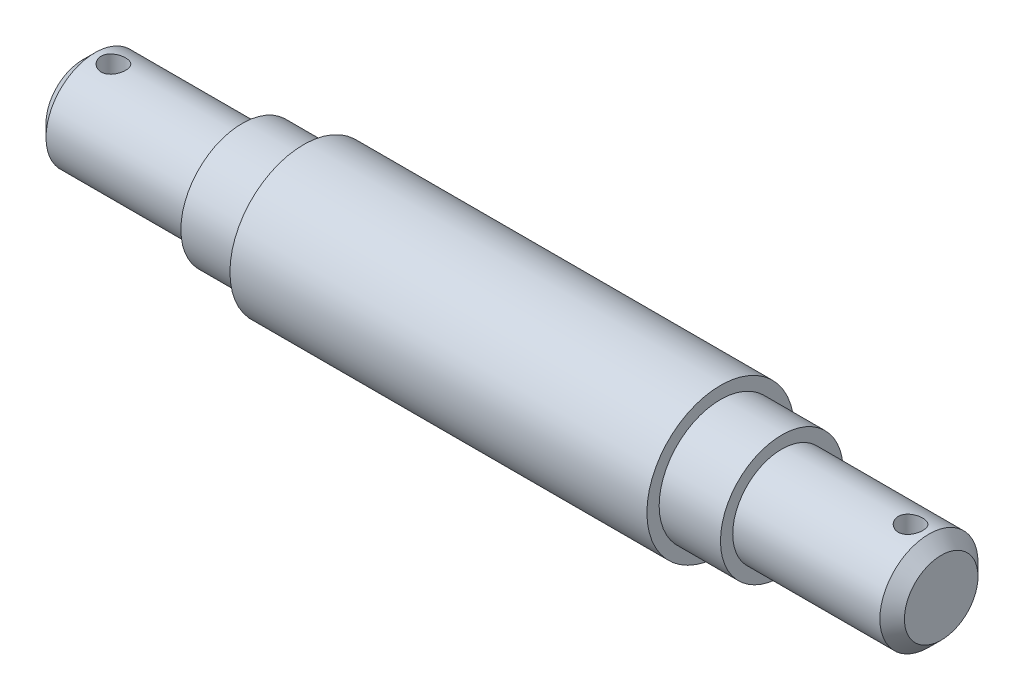
ISO-10303-21;
HEADER;
FILE_DESCRIPTION(('STEP AP214'),'2;1');
FILE_NAME('part.step','',(''),(''),'','','');
FILE_SCHEMA(('AUTOMOTIVE_DESIGN { 1 0 10303 214 1 1 1 1 }'));
ENDSEC;
DATA;
#1=APPLICATION_CONTEXT('core data for automotive mechanical design processes');
#2=APPLICATION_PROTOCOL_DEFINITION('international standard','automotive_design',2000,#1);
#3=PRODUCT_CONTEXT('',#1,'mechanical');
#4=PRODUCT('Part','Part','',(#3));
#5=PRODUCT_RELATED_PRODUCT_CATEGORY('part','',(#4));
#6=PRODUCT_DEFINITION_FORMATION('','',#4);
#7=PRODUCT_DEFINITION_CONTEXT('part definition',#1,'design');
#8=PRODUCT_DEFINITION('design','',#6,#7);
#9=PRODUCT_DEFINITION_SHAPE('','',#8);
#10=(LENGTH_UNIT() NAMED_UNIT(*) SI_UNIT(.MILLI.,.METRE.));
#11=(NAMED_UNIT(*) PLANE_ANGLE_UNIT() SI_UNIT($,.RADIAN.));
#12=(NAMED_UNIT(*) SI_UNIT($,.STERADIAN.) SOLID_ANGLE_UNIT());
#13=UNCERTAINTY_MEASURE_WITH_UNIT(LENGTH_MEASURE(1.E-05),#10,'distance_accuracy_value','');
#14=(GEOMETRIC_REPRESENTATION_CONTEXT(3) GLOBAL_UNCERTAINTY_ASSIGNED_CONTEXT((#13)) GLOBAL_UNIT_ASSIGNED_CONTEXT((#10,
#11,#12)) REPRESENTATION_CONTEXT('',''));
#15=CARTESIAN_POINT('',(0.,0.,0.));
#16=DIRECTION('',(0.,0.,1.));
#17=DIRECTION('',(1.,0.,0.));
#18=AXIS2_PLACEMENT_3D('',#15,#16,#17);
#19=CARTESIAN_POINT('',(0.,-4.,0.));
#20=DIRECTION('',(-1.,0.,0.));
#21=DIRECTION('',(0.,0.,1.));
#22=AXIS2_PLACEMENT_3D('',#19,#20,#21);
#23=PLANE('',#22);
#24=CARTESIAN_POINT('',(0.,0.,0.));
#25=DIRECTION('',(-1.,0.,0.));
#26=DIRECTION('',(0.,0.,1.));
#27=AXIS2_PLACEMENT_3D('',#24,#25,#26);
#28=CIRCLE('',#27,3.);
#29=CARTESIAN_POINT('',(0.,0.,3.));
#30=VERTEX_POINT('',#29);
#31=EDGE_CURVE('E60',#30,#30,#28,.T.);
#32=ORIENTED_EDGE('',*,*,#31,.T.);
#33=EDGE_LOOP('',(#32));
#34=FACE_BOUND('',#33,.T.);
#35=ADVANCED_FACE('F41',(#34),#23,.T.);
#36=CARTESIAN_POINT('',(70.,0.,0.));
#37=DIRECTION('',(1.,0.,0.));
#38=DIRECTION('',(0.,0.,-1.));
#39=AXIS2_PLACEMENT_3D('',#36,#37,#38);
#40=PLANE('',#39);
#41=CARTESIAN_POINT('',(70.,0.,0.));
#42=DIRECTION('',(1.,0.,0.));
#43=DIRECTION('',(0.,0.,-1.));
#44=AXIS2_PLACEMENT_3D('',#41,#42,#43);
#45=CIRCLE('',#44,3.);
#46=CARTESIAN_POINT('',(70.,0.,-3.));
#47=VERTEX_POINT('',#46);
#48=EDGE_CURVE('E10',#47,#47,#45,.T.);
#49=ORIENTED_EDGE('',*,*,#48,.T.);
#50=EDGE_LOOP('',(#49));
#51=FACE_BOUND('',#50,.T.);
#52=ADVANCED_FACE('F132',(#51),#40,.T.);
#53=CARTESIAN_POINT('',(0.,0.,0.));
#54=DIRECTION('',(-1.,0.,0.));
#55=DIRECTION('',(0.,0.,1.));
#56=AXIS2_PLACEMENT_3D('',#53,#54,#55);
#57=CYLINDRICAL_SURFACE('',#56,4.);
#58=CARTESIAN_POINT('',(69.,0.,0.));
#59=DIRECTION('',(1.,0.,0.));
#60=DIRECTION('',(0.,0.,-1.));
#61=AXIS2_PLACEMENT_3D('',#58,#59,#60);
#62=CIRCLE('',#61,4.);
#63=CARTESIAN_POINT('',(69.,0.,-4.));
#64=VERTEX_POINT('',#63);
#65=EDGE_CURVE('E47',#64,#64,#62,.F.);
#66=ORIENTED_EDGE('',*,*,#65,.T.);
#67=EDGE_LOOP('',(#66));
#68=FACE_BOUND('',#67,.T.);
#69=CARTESIAN_POINT('',(67.5,-3.87298334620742,0.999999999999998));
#70=CARTESIAN_POINT('',(67.4447796996432,-3.87298440057185,0.999998431438697));
#71=CARTESIAN_POINT('',(67.3895420405686,-3.87417722499279,0.995410498208067));
#72=CARTESIAN_POINT('',(67.2806529687674,-3.87880744892249,0.977209250194444));
#73=CARTESIAN_POINT('',(67.22700249822,-3.88224615474181,0.963590682698076));
#74=CARTESIAN_POINT('',(67.1228785847122,-3.89095489813012,0.927796479849631));
#75=CARTESIAN_POINT('',(67.0724011378422,-3.8962225706936,0.905631891140939));
#76=CARTESIAN_POINT('',(66.9758756589875,-3.90799276818327,0.853408456505401));
#77=CARTESIAN_POINT('',(66.9298278151688,-3.91449534553241,0.823349275424499));
#78=CARTESIAN_POINT('',(66.8424553418942,-3.92816286540368,0.755483370924512));
#79=CARTESIAN_POINT('',(66.8012425598597,-3.93533839048709,0.717534755081553));
#80=CARTESIAN_POINT('',(66.7256954422561,-3.94945150206622,0.635272825640327));
#81=CARTESIAN_POINT('',(66.6913617497514,-3.95638906626691,0.590958917672139));
#82=CARTESIAN_POINT('',(66.6300898129474,-3.96936166208095,0.496458080431564));
#83=CARTESIAN_POINT('',(66.6032614447354,-3.975382749602,0.446197830478043));
#84=CARTESIAN_POINT('',(66.5584761423388,-3.98572324770431,0.341705273717105));
#85=CARTESIAN_POINT('',(66.5405178992338,-3.99004290933748,0.28747355431677));
#86=CARTESIAN_POINT('',(66.5143408661686,-3.99641903539263,0.177743503501654));
#87=CARTESIAN_POINT('',(66.5059321422694,-3.99851957537723,0.122293087819583));
#88=CARTESIAN_POINT('',(66.4984966482898,-4.00037437642922,0.0107315277051037));
#89=CARTESIAN_POINT('',(66.4994684911162,-4.00012898438682,-0.0453795178152308));
#90=CARTESIAN_POINT('',(66.5106299401001,-3.99735237981413,-0.15535224717239));
#91=CARTESIAN_POINT('',(66.5206145300216,-3.9948720093635,-0.20923621560107));
#92=CARTESIAN_POINT('',(66.5491885080194,-3.98796334609942,-0.314538247413689));
#93=CARTESIAN_POINT('',(66.567778354151,-3.98353494959376,-0.365956179370442));
#94=CARTESIAN_POINT('',(66.6132010282748,-3.97315003880358,-0.465406703501811));
#95=CARTESIAN_POINT('',(66.6401068178647,-3.96718007878021,-0.513404509766509));
#96=CARTESIAN_POINT('',(66.7013422716465,-3.9543596152386,-0.604275622340492));
#97=CARTESIAN_POINT('',(66.7356732274243,-3.94750895860996,-0.647148035085508));
#98=CARTESIAN_POINT('',(66.811883496793,-3.93345485507808,-0.72777403508496));
#99=CARTESIAN_POINT('',(66.8539419569391,-3.92624687810367,-0.765357679075204));
#100=CARTESIAN_POINT('',(66.9438399894161,-3.91246017406683,-0.832976375963023));
#101=CARTESIAN_POINT('',(66.9916798317964,-3.90588147642388,-0.863011076046019));
#102=CARTESIAN_POINT('',(67.0921160136596,-3.89408198732659,-0.9147881290226));
#103=CARTESIAN_POINT('',(67.1447342921253,-3.88886793490288,-0.936489566970494));
#104=CARTESIAN_POINT('',(67.2530341872306,-3.88047456055983,-0.970685620636343));
#105=CARTESIAN_POINT('',(67.3087151455933,-3.87729480324087,-0.983182206552911));
#106=CARTESIAN_POINT('',(67.4199838006093,-3.87342142415656,-0.998331855466069));
#107=CARTESIAN_POINT('',(67.4755351173319,-3.87266435637459,-1.00123618956785));
#108=CARTESIAN_POINT('',(67.5863287746313,-3.87354937392416,-0.997806796206216));
#109=CARTESIAN_POINT('',(67.6415711431805,-3.87519123840507,-0.991473919139517));
#110=CARTESIAN_POINT('',(67.7492457059819,-3.88062832781824,-0.969970185575061));
#111=CARTESIAN_POINT('',(67.8017090906283,-3.8843878809375,-0.954945627312696));
#112=CARTESIAN_POINT('',(67.9033725831407,-3.89360287308385,-0.916647232668246));
#113=CARTESIAN_POINT('',(67.9525723036221,-3.89905851299446,-0.893372419085015));
#114=CARTESIAN_POINT('',(68.0473765111469,-3.91118454837305,-0.83870826717462));
#115=CARTESIAN_POINT('',(68.0928915360172,-3.91787667442657,-0.80716870153425));
#116=CARTESIAN_POINT('',(68.1780753451205,-3.93166833228686,-0.737060292934454));
#117=CARTESIAN_POINT('',(68.21774316666,-3.93876793091388,-0.698490294805437));
#118=CARTESIAN_POINT('',(68.2911244170284,-3.95278961212643,-0.614262720984723));
#119=CARTESIAN_POINT('',(68.3246640250195,-3.95970280824734,-0.568451952531591));
#120=CARTESIAN_POINT('',(68.3835743467805,-3.97238886645494,-0.471702682694674));
#121=CARTESIAN_POINT('',(68.4089454866433,-3.97816178801584,-0.42076444895759));
#122=CARTESIAN_POINT('',(68.4505784138112,-3.98788046295326,-0.315558201731088));
#123=CARTESIAN_POINT('',(68.4669057137516,-3.99183932008964,-0.261317381027879));
#124=CARTESIAN_POINT('',(68.4901841338434,-3.99754117358315,-0.150749760318804));
#125=CARTESIAN_POINT('',(68.4971370634956,-3.99928459757364,-0.0944233650412395));
#126=CARTESIAN_POINT('',(68.5013675895755,-4.00034169408811,0.0170835264433306));
#127=CARTESIAN_POINT('',(68.4989017090954,-3.99971978880008,0.0722538269660375));
#128=CARTESIAN_POINT('',(68.4849521727057,-3.99625896457423,0.181367496414744));
#129=CARTESIAN_POINT('',(68.4734687849869,-3.99342011157095,0.235310901780891));
#130=CARTESIAN_POINT('',(68.4419477802291,-3.98585432853963,0.34017103564482));
#131=CARTESIAN_POINT('',(68.4219565466854,-3.98113764502669,0.391102494581023));
#132=CARTESIAN_POINT('',(68.3740294209807,-3.97031288913382,0.488917053041472));
#133=CARTESIAN_POINT('',(68.3460925273304,-3.96420464137727,0.535799641265055));
#134=CARTESIAN_POINT('',(68.2822847660029,-3.95107249681342,0.625401928423903));
#135=CARTESIAN_POINT('',(68.2462398570926,-3.94403016945647,0.667994988300589));
#136=CARTESIAN_POINT('',(68.1675771480262,-3.92990649053207,0.746615020271253));
#137=CARTESIAN_POINT('',(68.1249576839021,-3.92282512952424,0.782640325068179));
#138=CARTESIAN_POINT('',(68.0333985857987,-3.90927475860683,0.847762026479241));
#139=CARTESIAN_POINT('',(67.9843558765875,-3.90281963730391,0.876716619446593));
#140=CARTESIAN_POINT('',(67.8819445100771,-3.8914395555011,0.925926896615621));
#141=CARTESIAN_POINT('',(67.8285790338927,-3.88651348244814,0.946188909759556));
#142=CARTESIAN_POINT('',(67.7294229881737,-3.87951908741315,0.97442252856557));
#143=CARTESIAN_POINT('',(67.6841068356177,-3.87708663005761,0.983993170595826));
#144=CARTESIAN_POINT('',(67.5925311309985,-3.87381838580358,0.996782292572817));
#145=CARTESIAN_POINT('',(67.5462716597494,-3.87298246270639,1.00000131437052));
#146=CARTESIAN_POINT('',(67.5,-3.87298334620742,0.999999999999998));
#147=B_SPLINE_CURVE_WITH_KNOTS('',3,(#69,#70,#71,#72,#73,#74,#75,#76,#77,#78,#79,#80,#81,#82,
#83,#84,#85,#86,#87,#88,#89,#90,#91,#92,#93,#94,#95,#96,#97,#98,#99,#100,#101,#102,#103,#104,
#105,#106,#107,#108,#109,#110,#111,#112,#113,#114,#115,#116,#117,#118,#119,#120,#121,#122,#123,
#124,#125,#126,#127,#128,#129,#130,#131,#132,#133,#134,#135,#136,#137,#138,#139,#140,#141,#142,
#143,#144,#145,#146),.UNSPECIFIED.,.T.,.F.,(4,2,2,2,2,2,2,2,2,2,2,2,2,2,2,2,2,2,2,2,2,2,2,2,2,2,
2,2,2,2,2,2,2,2,2,2,2,2,4),(0.,0.165490976675223,0.331078296534215,0.496452290829154,
0.661833306984669,0.830495816734641,0.999174085882202,1.17020598555443,1.34121263935112,
1.50875500394413,1.67627259462682,1.84007305071853,2.00388222686189,2.16917149698053,
2.33448954183839,2.50428186625039,2.67408212476195,2.84470572799637,3.01529280048094,
3.18137429900961,3.34744050869796,3.51078961999956,3.6741580856484,3.84073138339936,
4.00733207550291,4.17810132382401,4.34886166284094,4.51836829119045,4.68784219559889,
4.85273378447256,5.01762046947066,5.18161950620158,5.34563922291503,5.51358838629102,
5.68158012622477,5.85270590910144,6.02370688542921,6.16239130867204,6.30106390036081),.UNSPECIFIED.);
#148=CARTESIAN_POINT('',(67.5,-3.87298334620742,0.999999999999998));
#149=VERTEX_POINT('',#148);
#150=EDGE_CURVE('E62',#149,#149,#147,.T.);
#151=ORIENTED_EDGE('',*,*,#150,.F.);
#152=EDGE_LOOP('',(#151));
#153=FACE_BOUND('',#152,.T.);
#154=CARTESIAN_POINT('',(67.5,3.87298334620742,0.999999999999998));
#155=CARTESIAN_POINT('',(67.5552203003568,3.87298440057185,0.999998431438697));
#156=CARTESIAN_POINT('',(67.6104579594314,3.87417722499279,0.995410498208067));
#157=CARTESIAN_POINT('',(67.7193470312326,3.87880744892249,0.977209250194444));
#158=CARTESIAN_POINT('',(67.77299750178,3.88224615474181,0.963590682698076));
#159=CARTESIAN_POINT('',(67.8771214152878,3.89095489813012,0.927796479849631));
#160=CARTESIAN_POINT('',(67.9275988621578,3.8962225706936,0.905631891140939));
#161=CARTESIAN_POINT('',(68.0241243410125,3.90799276818327,0.853408456505401));
#162=CARTESIAN_POINT('',(68.0701721848312,3.91449534553241,0.823349275424499));
#163=CARTESIAN_POINT('',(68.1575446581058,3.92816286540368,0.755483370924512));
#164=CARTESIAN_POINT('',(68.1987574401403,3.93533839048709,0.717534755081553));
#165=CARTESIAN_POINT('',(68.2743045577439,3.94945150206622,0.635272825640327));
#166=CARTESIAN_POINT('',(68.3086382502486,3.95638906626691,0.590958917672139));
#167=CARTESIAN_POINT('',(68.3699101870526,3.96936166208095,0.496458080431564));
#168=CARTESIAN_POINT('',(68.3967385552646,3.975382749602,0.446197830478043));
#169=CARTESIAN_POINT('',(68.4415238576612,3.98572324770431,0.341705273717105));
#170=CARTESIAN_POINT('',(68.4594821007662,3.99004290933748,0.28747355431677));
#171=CARTESIAN_POINT('',(68.4856591338314,3.99641903539263,0.177743503501654));
#172=CARTESIAN_POINT('',(68.4940678577306,3.99851957537723,0.122293087819583));
#173=CARTESIAN_POINT('',(68.5015033517102,4.00037437642922,0.0107315277051038));
#174=CARTESIAN_POINT('',(68.5005315088838,4.00012898438682,-0.0453795178152307));
#175=CARTESIAN_POINT('',(68.4893700598999,3.99735237981413,-0.15535224717239));
#176=CARTESIAN_POINT('',(68.4793854699785,3.9948720093635,-0.20923621560107));
#177=CARTESIAN_POINT('',(68.4508114919806,3.98796334609942,-0.314538247413689));
#178=CARTESIAN_POINT('',(68.432221645849,3.98353494959376,-0.365956179370441));
#179=CARTESIAN_POINT('',(68.3867989717252,3.97315003880358,-0.465406703501808));
#180=CARTESIAN_POINT('',(68.3598931821353,3.96718007878021,-0.513404509766505));
#181=CARTESIAN_POINT('',(68.2986577283535,3.9543596152386,-0.604275622340489));
#182=CARTESIAN_POINT('',(68.2643267725758,3.94750895860996,-0.647148035085506));
#183=CARTESIAN_POINT('',(68.1881165032071,3.93345485507808,-0.727774035084959));
#184=CARTESIAN_POINT('',(68.1460580430609,3.92624687810367,-0.765357679075204));
#185=CARTESIAN_POINT('',(68.0561600105839,3.91246017406682,-0.832976375963023));
#186=CARTESIAN_POINT('',(68.0083201682036,3.90588147642388,-0.863011076046019));
#187=CARTESIAN_POINT('',(67.9078839863404,3.89408198732659,-0.914788129022598));
#188=CARTESIAN_POINT('',(67.8552657078747,3.88886793490288,-0.936489566970491));
#189=CARTESIAN_POINT('',(67.7469658127694,3.88047456055983,-0.970685620636341));
#190=CARTESIAN_POINT('',(67.6912848544067,3.87729480324087,-0.98318220655291));
#191=CARTESIAN_POINT('',(67.5800161993907,3.87342142415656,-0.998331855466069));
#192=CARTESIAN_POINT('',(67.5244648826681,3.87266435637459,-1.00123618956785));
#193=CARTESIAN_POINT('',(67.4136712253687,3.87354937392416,-0.997806796206216));
#194=CARTESIAN_POINT('',(67.3584288568195,3.87519123840507,-0.991473919139516));
#195=CARTESIAN_POINT('',(67.2507542940181,3.88062832781824,-0.96997018557506));
#196=CARTESIAN_POINT('',(67.1982909093717,3.8843878809375,-0.954945627312694));
#197=CARTESIAN_POINT('',(67.0966274168593,3.89360287308385,-0.916647232668243));
#198=CARTESIAN_POINT('',(67.0474276963779,3.89905851299446,-0.893372419085012));
#199=CARTESIAN_POINT('',(66.9526234888531,3.91118454837305,-0.83870826717462));
#200=CARTESIAN_POINT('',(66.9071084639828,3.91787667442657,-0.80716870153425));
#201=CARTESIAN_POINT('',(66.8219246548795,3.93166833228686,-0.737060292934454));
#202=CARTESIAN_POINT('',(66.78225683334,3.93876793091388,-0.698490294805437));
#203=CARTESIAN_POINT('',(66.7088755829716,3.95278961212643,-0.614262720984723));
#204=CARTESIAN_POINT('',(66.6753359749805,3.95970280824734,-0.568451952531591));
#205=CARTESIAN_POINT('',(66.6164256532195,3.97238886645494,-0.471702682694674));
#206=CARTESIAN_POINT('',(66.5910545133567,3.97816178801584,-0.42076444895759));
#207=CARTESIAN_POINT('',(66.5494215861888,3.98788046295326,-0.315558201731088));
#208=CARTESIAN_POINT('',(66.5330942862484,3.99183932008964,-0.261317381027879));
#209=CARTESIAN_POINT('',(66.5098158661566,3.99754117358315,-0.150749760318804));
#210=CARTESIAN_POINT('',(66.5028629365044,3.99928459757364,-0.0944233650412395));
#211=CARTESIAN_POINT('',(66.4986324104245,4.00034169408811,0.0170835264433306));
#212=CARTESIAN_POINT('',(66.5010982909046,3.99971978880008,0.0722538269660375));
#213=CARTESIAN_POINT('',(66.5150478272943,3.99625896457423,0.181367496414744));
#214=CARTESIAN_POINT('',(66.5265312150131,3.99342011157095,0.235310901780891));
#215=CARTESIAN_POINT('',(66.5580522197709,3.98585432853963,0.34017103564482));
#216=CARTESIAN_POINT('',(66.5780434533146,3.98113764502669,0.391102494581023));
#217=CARTESIAN_POINT('',(66.6259705790193,3.97031288913382,0.488917053041472));
#218=CARTESIAN_POINT('',(66.6539074726696,3.96420464137727,0.535799641265055));
#219=CARTESIAN_POINT('',(66.7177152339971,3.95107249681342,0.625401928423903));
#220=CARTESIAN_POINT('',(66.7537601429074,3.94403016945647,0.667994988300589));
#221=CARTESIAN_POINT('',(66.8324228519738,3.92990649053207,0.746615020271253));
#222=CARTESIAN_POINT('',(66.8750423160979,3.92282512952424,0.782640325068179));
#223=CARTESIAN_POINT('',(66.9666014142013,3.90927475860683,0.847762026479241));
#224=CARTESIAN_POINT('',(67.0156441234125,3.90281963730391,0.876716619446593));
#225=CARTESIAN_POINT('',(67.1180554899229,3.8914395555011,0.925926896615621));
#226=CARTESIAN_POINT('',(67.1714209661073,3.88651348244814,0.946188909759556));
#227=CARTESIAN_POINT('',(67.2705770118263,3.87951908741315,0.97442252856557));
#228=CARTESIAN_POINT('',(67.3158931643824,3.87708663005761,0.983993170595826));
#229=CARTESIAN_POINT('',(67.4074688690015,3.87381838580358,0.996782292572817));
#230=CARTESIAN_POINT('',(67.4537283402506,3.87298246270639,1.00000131437052));
#231=CARTESIAN_POINT('',(67.5,3.87298334620742,0.999999999999998));
#232=B_SPLINE_CURVE_WITH_KNOTS('',3,(#154,#155,#156,#157,#158,#159,#160,#161,#162,#163,#164,
#165,#166,#167,#168,#169,#170,#171,#172,#173,#174,#175,#176,#177,#178,#179,#180,#181,#182,#183,
#184,#185,#186,#187,#188,#189,#190,#191,#192,#193,#194,#195,#196,#197,#198,#199,#200,#201,#202,
#203,#204,#205,#206,#207,#208,#209,#210,#211,#212,#213,#214,#215,#216,#217,#218,#219,#220,#221,
#222,#223,#224,#225,#226,#227,#228,#229,#230,#231),.UNSPECIFIED.,.T.,.F.,(4,2,2,2,2,2,2,2,2,2,2,
2,2,2,2,2,2,2,2,2,2,2,2,2,2,2,2,2,2,2,2,2,2,2,2,2,2,2,4),(0.,0.165490976675223,
0.331078296534215,0.496452290829154,0.661833306984669,0.830495816734641,0.999174085882202,
1.17020598555443,1.34121263935112,1.50875500394413,1.67627259462682,1.84007305071853,
2.00388222686189,2.16917149698051,2.33448954183839,2.50428186625039,2.67408212476196,
2.84470572799636,3.01529280048094,3.18137429900961,3.34744050869796,3.51078961999957,
3.6741580856484,3.84073138339937,4.00733207550291,4.17810132382402,4.34886166284095,
4.51836829119045,4.68784219559889,4.85273378447256,5.01762046947066,5.18161950620158,
5.34563922291503,5.51358838629102,5.68158012622477,5.85270590910144,6.02370688542921,
6.16239130867204,6.30106390036081),.UNSPECIFIED.);
#233=CARTESIAN_POINT('',(67.5,3.87298334620742,0.999999999999998));
#234=VERTEX_POINT('',#233);
#235=EDGE_CURVE('E75',#234,#234,#232,.T.);
#236=ORIENTED_EDGE('',*,*,#235,.F.);
#237=EDGE_LOOP('',(#236));
#238=FACE_BOUND('',#237,.T.);
#239=CARTESIAN_POINT('',(57.,0.,0.));
#240=DIRECTION('',(-1.,0.,0.));
#241=DIRECTION('',(0.,0.,1.));
#242=AXIS2_PLACEMENT_3D('',#239,#240,#241);
#243=CIRCLE('',#242,4.);
#244=CARTESIAN_POINT('',(57.,0.,4.));
#245=VERTEX_POINT('',#244);
#246=EDGE_CURVE('E64',#245,#245,#243,.T.);
#247=ORIENTED_EDGE('',*,*,#246,.F.);
#248=EDGE_LOOP('',(#247));
#249=FACE_BOUND('',#248,.T.);
#250=ADVANCED_FACE('F79',(#68,#153,#238,#249),#57,.T.);
#251=CARTESIAN_POINT('',(57.,-4.,0.));
#252=DIRECTION('',(1.,0.,0.));
#253=DIRECTION('',(0.,0.,-1.));
#254=AXIS2_PLACEMENT_3D('',#251,#252,#253);
#255=PLANE('',#254);
#256=ORIENTED_EDGE('',*,*,#246,.T.);
#257=EDGE_LOOP('',(#256));
#258=FACE_BOUND('',#257,.T.);
#259=CARTESIAN_POINT('',(57.,0.,0.));
#260=DIRECTION('',(-1.,0.,0.));
#261=DIRECTION('',(0.,0.,1.));
#262=AXIS2_PLACEMENT_3D('',#259,#260,#261);
#263=CIRCLE('',#262,5.);
#264=CARTESIAN_POINT('',(57.,0.,5.));
#265=VERTEX_POINT('',#264);
#266=EDGE_CURVE('E262',#265,#265,#263,.T.);
#267=ORIENTED_EDGE('',*,*,#266,.F.);
#268=EDGE_LOOP('',(#267));
#269=FACE_BOUND('',#268,.T.);
#270=ADVANCED_FACE('F227',(#258,#269),#255,.T.);
#271=CARTESIAN_POINT('',(0.,0.,0.));
#272=DIRECTION('',(-1.,0.,0.));
#273=DIRECTION('',(0.,0.,1.));
#274=AXIS2_PLACEMENT_3D('',#271,#272,#273);
#275=CYLINDRICAL_SURFACE('',#274,5.);
#276=ORIENTED_EDGE('',*,*,#266,.T.);
#277=EDGE_LOOP('',(#276));
#278=FACE_BOUND('',#277,.T.);
#279=CARTESIAN_POINT('',(52.,0.,0.));
#280=DIRECTION('',(-1.,0.,0.));
#281=DIRECTION('',(0.,0.,1.));
#282=AXIS2_PLACEMENT_3D('',#279,#280,#281);
#283=CIRCLE('',#282,5.);
#284=CARTESIAN_POINT('',(52.,0.,5.));
#285=VERTEX_POINT('',#284);
#286=EDGE_CURVE('E266',#285,#285,#283,.T.);
#287=ORIENTED_EDGE('',*,*,#286,.F.);
#288=EDGE_LOOP('',(#287));
#289=FACE_BOUND('',#288,.T.);
#290=ADVANCED_FACE('F217',(#278,#289),#275,.T.);
#291=CARTESIAN_POINT('',(52.,-5.,0.));
#292=DIRECTION('',(1.,0.,0.));
#293=DIRECTION('',(0.,0.,-1.));
#294=AXIS2_PLACEMENT_3D('',#291,#292,#293);
#295=PLANE('',#294);
#296=ORIENTED_EDGE('',*,*,#286,.T.);
#297=EDGE_LOOP('',(#296));
#298=FACE_BOUND('',#297,.T.);
#299=CARTESIAN_POINT('',(52.,0.,0.));
#300=DIRECTION('',(-1.,0.,0.));
#301=DIRECTION('',(0.,0.,1.));
#302=AXIS2_PLACEMENT_3D('',#299,#300,#301);
#303=CIRCLE('',#302,6.);
#304=CARTESIAN_POINT('',(52.,0.,6.));
#305=VERTEX_POINT('',#304);
#306=EDGE_CURVE('E271',#305,#305,#303,.T.);
#307=ORIENTED_EDGE('',*,*,#306,.F.);
#308=EDGE_LOOP('',(#307));
#309=FACE_BOUND('',#308,.T.);
#310=ADVANCED_FACE('F208',(#298,#309),#295,.T.);
#311=CARTESIAN_POINT('',(0.,0.,0.));
#312=DIRECTION('',(-1.,0.,0.));
#313=DIRECTION('',(0.,0.,1.));
#314=AXIS2_PLACEMENT_3D('',#311,#312,#313);
#315=CYLINDRICAL_SURFACE('',#314,6.00000000000001);
#316=ORIENTED_EDGE('',*,*,#306,.T.);
#317=EDGE_LOOP('',(#316));
#318=FACE_BOUND('',#317,.T.);
#319=CARTESIAN_POINT('',(18.,0.,0.));
#320=DIRECTION('',(-1.,0.,0.));
#321=DIRECTION('',(0.,0.,1.));
#322=AXIS2_PLACEMENT_3D('',#319,#320,#321);
#323=CIRCLE('',#322,6.00000000000001);
#324=CARTESIAN_POINT('',(18.,0.,6.00000000000001));
#325=VERTEX_POINT('',#324);
#326=EDGE_CURVE('E273',#325,#325,#323,.T.);
#327=ORIENTED_EDGE('',*,*,#326,.F.);
#328=EDGE_LOOP('',(#327));
#329=FACE_BOUND('',#328,.T.);
#330=ADVANCED_FACE('F196',(#318,#329),#315,.T.);
#331=CARTESIAN_POINT('',(18.,-6.00000000000001,0.));
#332=DIRECTION('',(-1.,0.,0.));
#333=DIRECTION('',(0.,0.,1.));
#334=AXIS2_PLACEMENT_3D('',#331,#332,#333);
#335=PLANE('',#334);
#336=ORIENTED_EDGE('',*,*,#326,.T.);
#337=EDGE_LOOP('',(#336));
#338=FACE_BOUND('',#337,.T.);
#339=CARTESIAN_POINT('',(18.,0.,0.));
#340=DIRECTION('',(-1.,0.,0.));
#341=DIRECTION('',(0.,0.,1.));
#342=AXIS2_PLACEMENT_3D('',#339,#340,#341);
#343=CIRCLE('',#342,5.);
#344=CARTESIAN_POINT('',(18.,0.,5.));
#345=VERTEX_POINT('',#344);
#346=EDGE_CURVE('E280',#345,#345,#343,.T.);
#347=ORIENTED_EDGE('',*,*,#346,.F.);
#348=EDGE_LOOP('',(#347));
#349=FACE_BOUND('',#348,.T.);
#350=ADVANCED_FACE('F126',(#338,#349),#335,.T.);
#351=CARTESIAN_POINT('',(0.,0.,0.));
#352=DIRECTION('',(-1.,0.,0.));
#353=DIRECTION('',(0.,0.,1.));
#354=AXIS2_PLACEMENT_3D('',#351,#352,#353);
#355=CYLINDRICAL_SURFACE('',#354,5.);
#356=ORIENTED_EDGE('',*,*,#346,.T.);
#357=EDGE_LOOP('',(#356));
#358=FACE_BOUND('',#357,.T.);
#359=CARTESIAN_POINT('',(13.,0.,0.));
#360=DIRECTION('',(-1.,0.,0.));
#361=DIRECTION('',(0.,0.,1.));
#362=AXIS2_PLACEMENT_3D('',#359,#360,#361);
#363=CIRCLE('',#362,5.);
#364=CARTESIAN_POINT('',(13.,0.,5.));
#365=VERTEX_POINT('',#364);
#366=EDGE_CURVE('E109',#365,#365,#363,.T.);
#367=ORIENTED_EDGE('',*,*,#366,.F.);
#368=EDGE_LOOP('',(#367));
#369=FACE_BOUND('',#368,.T.);
#370=ADVANCED_FACE('F125',(#358,#369),#355,.T.);
#371=CARTESIAN_POINT('',(13.,-5.,0.));
#372=DIRECTION('',(-1.,0.,0.));
#373=DIRECTION('',(0.,0.,1.));
#374=AXIS2_PLACEMENT_3D('',#371,#372,#373);
#375=PLANE('',#374);
#376=ORIENTED_EDGE('',*,*,#366,.T.);
#377=EDGE_LOOP('',(#376));
#378=FACE_BOUND('',#377,.T.);
#379=CARTESIAN_POINT('',(13.,0.,0.));
#380=DIRECTION('',(-1.,0.,0.));
#381=DIRECTION('',(0.,0.,1.));
#382=AXIS2_PLACEMENT_3D('',#379,#380,#381);
#383=CIRCLE('',#382,4.);
#384=CARTESIAN_POINT('',(13.,0.,4.));
#385=VERTEX_POINT('',#384);
#386=EDGE_CURVE('E110',#385,#385,#383,.T.);
#387=ORIENTED_EDGE('',*,*,#386,.F.);
#388=EDGE_LOOP('',(#387));
#389=FACE_BOUND('',#388,.T.);
#390=ADVANCED_FACE('F117',(#378,#389),#375,.T.);
#391=CARTESIAN_POINT('',(0.,0.,0.));
#392=DIRECTION('',(-1.,0.,0.));
#393=DIRECTION('',(0.,0.,1.));
#394=AXIS2_PLACEMENT_3D('',#391,#392,#393);
#395=CYLINDRICAL_SURFACE('',#394,4.);
#396=CARTESIAN_POINT('',(1.00000000000001,0.,0.));
#397=DIRECTION('',(-1.,0.,0.));
#398=DIRECTION('',(0.,0.,1.));
#399=AXIS2_PLACEMENT_3D('',#396,#397,#398);
#400=CIRCLE('',#399,4.);
#401=CARTESIAN_POINT('',(1.00000000000001,0.,4.));
#402=VERTEX_POINT('',#401);
#403=EDGE_CURVE('E52',#402,#402,#400,.F.);
#404=ORIENTED_EDGE('',*,*,#403,.T.);
#405=EDGE_LOOP('',(#404));
#406=FACE_BOUND('',#405,.T.);
#407=CARTESIAN_POINT('',(2.5,-3.87298334620742,1.));
#408=CARTESIAN_POINT('',(2.44477969964321,-3.87298440057185,0.999998431438699));
#409=CARTESIAN_POINT('',(2.38954204056864,-3.87417722499279,0.995410498208069));
#410=CARTESIAN_POINT('',(2.28065296876739,-3.87880744892249,0.977209250194446));
#411=CARTESIAN_POINT('',(2.22700249822003,-3.88224615474181,0.963590682698077));
#412=CARTESIAN_POINT('',(2.12287858471216,-3.89095489813012,0.927796479849635));
#413=CARTESIAN_POINT('',(2.07240113784224,-3.8962225706936,0.905631891140943));
#414=CARTESIAN_POINT('',(1.97587565898752,-3.90799276818327,0.853408456505407));
#415=CARTESIAN_POINT('',(1.92982781516885,-3.91449534553241,0.823349275424505));
#416=CARTESIAN_POINT('',(1.84245534189415,-3.92816286540368,0.755483370924517));
#417=CARTESIAN_POINT('',(1.80124255985972,-3.93533839048709,0.717534755081557));
#418=CARTESIAN_POINT('',(1.72569544225612,-3.94945150206622,0.635272825640328));
#419=CARTESIAN_POINT('',(1.69136174975137,-3.95638906626692,0.590958917672139));
#420=CARTESIAN_POINT('',(1.63008981294742,-3.96936166208095,0.496458080431564));
#421=CARTESIAN_POINT('',(1.60326144473539,-3.975382749602,0.446197830478043));
#422=CARTESIAN_POINT('',(1.55847614233879,-3.98572324770431,0.341705273717109));
#423=CARTESIAN_POINT('',(1.5405178992338,-3.99004290933748,0.287473554316777));
#424=CARTESIAN_POINT('',(1.51434086616856,-3.99641903539263,0.177743503501663));
#425=CARTESIAN_POINT('',(1.50593214226937,-3.99851957537723,0.122293087819589));
#426=CARTESIAN_POINT('',(1.49849664828978,-4.00037437642922,0.0107315277051073));
#427=CARTESIAN_POINT('',(1.49946849111616,-4.00012898438682,-0.045379517815228));
#428=CARTESIAN_POINT('',(1.51062994010006,-3.99735237981413,-0.155352247172388));
#429=CARTESIAN_POINT('',(1.52061453002154,-3.9948720093635,-0.209236215601067));
#430=CARTESIAN_POINT('',(1.5491885080194,-3.98796334609942,-0.314538247413687));
#431=CARTESIAN_POINT('',(1.56777835415096,-3.98353494959377,-0.365956179370439));
#432=CARTESIAN_POINT('',(1.61320102827483,-3.97315003880358,-0.465406703501807));
#433=CARTESIAN_POINT('',(1.6401068178647,-3.96718007878022,-0.513404509766505));
#434=CARTESIAN_POINT('',(1.7013422716465,-3.9543596152386,-0.604275622340489));
#435=CARTESIAN_POINT('',(1.73567322742425,-3.94750895860996,-0.647148035085506));
#436=CARTESIAN_POINT('',(1.81188349679295,-3.93345485507808,-0.727774035084957));
#437=CARTESIAN_POINT('',(1.85394195693911,-3.92624687810367,-0.7653576790752));
#438=CARTESIAN_POINT('',(1.9438399894161,-3.91246017406683,-0.832976375963019));
#439=CARTESIAN_POINT('',(1.9916798317964,-3.90588147642388,-0.863011076046017));
#440=CARTESIAN_POINT('',(2.09211601365959,-3.89408198732659,-0.914788129022598));
#441=CARTESIAN_POINT('',(2.14473429212528,-3.88886793490288,-0.936489566970491));
#442=CARTESIAN_POINT('',(2.25303418723058,-3.88047456055983,-0.970685620636341));
#443=CARTESIAN_POINT('',(2.30871514559326,-3.87729480324088,-0.98318220655291));
#444=CARTESIAN_POINT('',(2.41998380060925,-3.87342142415656,-0.998331855466071));
#445=CARTESIAN_POINT('',(2.47553511733185,-3.87266435637459,-1.00123618956785));
#446=CARTESIAN_POINT('',(2.58632877463126,-3.87354937392416,-0.997806796206219));
#447=CARTESIAN_POINT('',(2.6415711431805,-3.87519123840507,-0.99147391913952));
#448=CARTESIAN_POINT('',(2.74924570598188,-3.88062832781824,-0.969970185575064));
#449=CARTESIAN_POINT('',(2.80170909062834,-3.8843878809375,-0.954945627312698));
#450=CARTESIAN_POINT('',(2.90337258314067,-3.89360287308385,-0.916647232668248));
#451=CARTESIAN_POINT('',(2.95257230362214,-3.89905851299446,-0.893372419085017));
#452=CARTESIAN_POINT('',(3.04737651114694,-3.91118454837305,-0.838708267174622));
#453=CARTESIAN_POINT('',(3.09289153601724,-3.91787667442657,-0.807168701534251));
#454=CARTESIAN_POINT('',(3.17807534512054,-3.93166833228687,-0.737060292934455));
#455=CARTESIAN_POINT('',(3.21774316666003,-3.93876793091388,-0.698490294805439));
#456=CARTESIAN_POINT('',(3.29112441702838,-3.95278961212643,-0.614262720984725));
#457=CARTESIAN_POINT('',(3.32466402501953,-3.95970280824734,-0.568451952531592));
#458=CARTESIAN_POINT('',(3.3835743467805,-3.97238886645494,-0.471702682694674));
#459=CARTESIAN_POINT('',(3.40894548664328,-3.97816178801584,-0.42076444895759));
#460=CARTESIAN_POINT('',(3.45057841381117,-3.98788046295326,-0.315558201731089));
#461=CARTESIAN_POINT('',(3.46690571375163,-3.99183932008964,-0.26131738102788));
#462=CARTESIAN_POINT('',(3.49018413384337,-3.99754117358315,-0.150749760318806));
#463=CARTESIAN_POINT('',(3.49713706349562,-3.99928459757364,-0.0944233650412421));
#464=CARTESIAN_POINT('',(3.50136758957553,-4.00034169408811,0.0170835264433279));
#465=CARTESIAN_POINT('',(3.49890170909539,-3.99971978880009,0.0722538269660349));
#466=CARTESIAN_POINT('',(3.48495217270567,-3.99625896457424,0.181367496414741));
#467=CARTESIAN_POINT('',(3.4734687849869,-3.99342011157095,0.235310901780888));
#468=CARTESIAN_POINT('',(3.44194778022907,-3.98585432853963,0.340171035644817));
#469=CARTESIAN_POINT('',(3.42195654668538,-3.98113764502669,0.39110249458102));
#470=CARTESIAN_POINT('',(3.37402942098067,-3.97031288913382,0.488917053041469));
#471=CARTESIAN_POINT('',(3.34609252733043,-3.96420464137727,0.535799641265052));
#472=CARTESIAN_POINT('',(3.28228476600293,-3.95107249681343,0.625401928423901));
#473=CARTESIAN_POINT('',(3.24623985709263,-3.94403016945647,0.667994988300588));
#474=CARTESIAN_POINT('',(3.16757714802619,-3.92990649053207,0.746615020271253));
#475=CARTESIAN_POINT('',(3.12495768390205,-3.92282512952424,0.782640325068179));
#476=CARTESIAN_POINT('',(3.0333985857987,-3.90927475860683,0.847762026479241));
#477=CARTESIAN_POINT('',(2.98435587658752,-3.90281963730391,0.876716619446594));
#478=CARTESIAN_POINT('',(2.88194451007715,-3.8914395555011,0.925926896615622));
#479=CARTESIAN_POINT('',(2.82857903389271,-3.88651348244814,0.946188909759557));
#480=CARTESIAN_POINT('',(2.72942298817372,-3.87951908741315,0.974422528565572));
#481=CARTESIAN_POINT('',(2.68410683561764,-3.87708663005761,0.983993170595829));
#482=CARTESIAN_POINT('',(2.59253113099853,-3.87381838580358,0.996782292572819));
#483=CARTESIAN_POINT('',(2.54627165974937,-3.87298246270639,1.00000131437052));
#484=CARTESIAN_POINT('',(2.5,-3.87298334620742,1.));
#485=B_SPLINE_CURVE_WITH_KNOTS('',3,(#407,#408,#409,#410,#411,#412,#413,#414,#415,#416,#417,
#418,#419,#420,#421,#422,#423,#424,#425,#426,#427,#428,#429,#430,#431,#432,#433,#434,#435,#436,
#437,#438,#439,#440,#441,#442,#443,#444,#445,#446,#447,#448,#449,#450,#451,#452,#453,#454,#455,
#456,#457,#458,#459,#460,#461,#462,#463,#464,#465,#466,#467,#468,#469,#470,#471,#472,#473,#474,
#475,#476,#477,#478,#479,#480,#481,#482,#483,#484),.UNSPECIFIED.,.T.,.F.,(4,2,2,2,2,2,2,2,2,2,2,
2,2,2,2,2,2,2,2,2,2,2,2,2,2,2,2,2,2,2,2,2,2,2,2,2,2,2,4),(0.,0.16549097667523,0.331078296534211,
0.496452290829153,0.661833306984659,0.83049581673465,0.999174085882212,1.17020598555443,
1.34121263935111,1.50875500394413,1.67627259462683,1.84007305071853,2.00388222686189,
2.16917149698052,2.3344895418384,2.50428186625039,2.67408212476195,2.84470572799636,
3.01529280048094,3.18137429900961,3.34744050869795,3.51078961999957,3.67415808564842,
3.84073138339938,4.00733207550292,4.17810132382402,4.34886166284096,4.51836829119046,
4.6878421955989,4.85273378447257,5.01762046947067,5.18161950620159,5.34563922291504,
5.51358838629103,5.68158012622478,5.85270590910146,6.02370688542923,6.16239130867207,
6.30106390036083),.UNSPECIFIED.);
#486=CARTESIAN_POINT('',(2.5,-3.87298334620742,1.));
#487=VERTEX_POINT('',#486);
#488=EDGE_CURVE('E105',#487,#487,#485,.T.);
#489=ORIENTED_EDGE('',*,*,#488,.F.);
#490=EDGE_LOOP('',(#489));
#491=FACE_BOUND('',#490,.T.);
#492=CARTESIAN_POINT('',(2.5,3.87298334620742,1.));
#493=CARTESIAN_POINT('',(2.55522030035679,3.87298440057185,0.999998431438699));
#494=CARTESIAN_POINT('',(2.61045795943136,3.87417722499279,0.995410498208069));
#495=CARTESIAN_POINT('',(2.71934703123261,3.87880744892249,0.977209250194446));
#496=CARTESIAN_POINT('',(2.77299750177997,3.88224615474181,0.963590682698077));
#497=CARTESIAN_POINT('',(2.87712141528784,3.89095489813012,0.927796479849635));
#498=CARTESIAN_POINT('',(2.92759886215776,3.8962225706936,0.905631891140944));
#499=CARTESIAN_POINT('',(3.02412434101248,3.90799276818327,0.853408456505407));
#500=CARTESIAN_POINT('',(3.07017218483115,3.91449534553241,0.823349275424505));
#501=CARTESIAN_POINT('',(3.15754465810585,3.92816286540368,0.755483370924517));
#502=CARTESIAN_POINT('',(3.19875744014028,3.93533839048709,0.717534755081557));
#503=CARTESIAN_POINT('',(3.27430455774388,3.94945150206622,0.635272825640328));
#504=CARTESIAN_POINT('',(3.30863825024863,3.95638906626692,0.590958917672139));
#505=CARTESIAN_POINT('',(3.36991018705258,3.96936166208095,0.496458080431564));
#506=CARTESIAN_POINT('',(3.39673855526461,3.975382749602,0.446197830478043));
#507=CARTESIAN_POINT('',(3.44152385766121,3.98572324770431,0.341705273717109));
#508=CARTESIAN_POINT('',(3.4594821007662,3.99004290933748,0.287473554316777));
#509=CARTESIAN_POINT('',(3.48565913383144,3.99641903539263,0.177743503501663));
#510=CARTESIAN_POINT('',(3.49406785773063,3.99851957537723,0.122293087819589));
#511=CARTESIAN_POINT('',(3.50150335171022,4.00037437642922,0.0107315277051074));
#512=CARTESIAN_POINT('',(3.50053150888384,4.00012898438682,-0.0453795178152279));
#513=CARTESIAN_POINT('',(3.48937005989994,3.99735237981413,-0.155352247172388));
#514=CARTESIAN_POINT('',(3.47938546997846,3.9948720093635,-0.209236215601067));
#515=CARTESIAN_POINT('',(3.4508114919806,3.98796334609942,-0.314538247413687));
#516=CARTESIAN_POINT('',(3.43222164584904,3.98353494959377,-0.365956179370439));
#517=CARTESIAN_POINT('',(3.38679897172517,3.97315003880358,-0.465406703501807));
#518=CARTESIAN_POINT('',(3.3598931821353,3.96718007878022,-0.513404509766505));
#519=CARTESIAN_POINT('',(3.2986577283535,3.9543596152386,-0.604275622340489));
#520=CARTESIAN_POINT('',(3.26432677257575,3.94750895860996,-0.647148035085506));
#521=CARTESIAN_POINT('',(3.18811650320705,3.93345485507808,-0.727774035084957));
#522=CARTESIAN_POINT('',(3.14605804306089,3.92624687810367,-0.7653576790752));
#523=CARTESIAN_POINT('',(3.0561600105839,3.91246017406683,-0.832976375963019));
#524=CARTESIAN_POINT('',(3.0083201682036,3.90588147642388,-0.863011076046017));
#525=CARTESIAN_POINT('',(2.90788398634041,3.89408198732659,-0.914788129022598));
#526=CARTESIAN_POINT('',(2.85526570787472,3.88886793490288,-0.936489566970491));
#527=CARTESIAN_POINT('',(2.74696581276942,3.88047456055983,-0.970685620636341));
#528=CARTESIAN_POINT('',(2.69128485440675,3.87729480324088,-0.98318220655291));
#529=CARTESIAN_POINT('',(2.58001619939075,3.87342142415656,-0.998331855466071));
#530=CARTESIAN_POINT('',(2.52446488266815,3.87266435637459,-1.00123618956785));
#531=CARTESIAN_POINT('',(2.41367122536874,3.87354937392416,-0.997806796206219));
#532=CARTESIAN_POINT('',(2.3584288568195,3.87519123840507,-0.99147391913952));
#533=CARTESIAN_POINT('',(2.25075429401812,3.88062832781824,-0.969970185575065));
#534=CARTESIAN_POINT('',(2.19829090937166,3.8843878809375,-0.954945627312698));
#535=CARTESIAN_POINT('',(2.09662741685933,3.89360287308385,-0.916647232668248));
#536=CARTESIAN_POINT('',(2.04742769637786,3.89905851299446,-0.893372419085018));
#537=CARTESIAN_POINT('',(1.95262348885306,3.91118454837305,-0.838708267174623));
#538=CARTESIAN_POINT('',(1.90710846398276,3.91787667442657,-0.807168701534251));
#539=CARTESIAN_POINT('',(1.82192465487946,3.93166833228687,-0.737060292934456));
#540=CARTESIAN_POINT('',(1.78225683333997,3.93876793091388,-0.698490294805439));
#541=CARTESIAN_POINT('',(1.70887558297162,3.95278961212643,-0.614262720984726));
#542=CARTESIAN_POINT('',(1.67533597498047,3.95970280824734,-0.568451952531592));
#543=CARTESIAN_POINT('',(1.6164256532195,3.97238886645494,-0.471702682694675));
#544=CARTESIAN_POINT('',(1.59105451335672,3.97816178801584,-0.420764448957591));
#545=CARTESIAN_POINT('',(1.54942158618883,3.98788046295326,-0.31555820173109));
#546=CARTESIAN_POINT('',(1.53309428624838,3.99183932008964,-0.261317381027881));
#547=CARTESIAN_POINT('',(1.50981586615663,3.99754117358315,-0.150749760318808));
#548=CARTESIAN_POINT('',(1.50286293650438,3.99928459757364,-0.0944233650412432));
#549=CARTESIAN_POINT('',(1.49863241042447,4.00034169408811,0.0170835264433266));
#550=CARTESIAN_POINT('',(1.50109829090461,3.99971978880009,0.0722538269660332));
#551=CARTESIAN_POINT('',(1.51504782729433,3.99625896457424,0.18136749641474));
#552=CARTESIAN_POINT('',(1.5265312150131,3.99342011157095,0.235310901780887));
#553=CARTESIAN_POINT('',(1.55805221977093,3.98585432853963,0.340171035644817));
#554=CARTESIAN_POINT('',(1.57804345331462,3.98113764502669,0.39110249458102));
#555=CARTESIAN_POINT('',(1.62597057901933,3.97031288913382,0.488917053041469));
#556=CARTESIAN_POINT('',(1.65390747266957,3.96420464137727,0.535799641265051));
#557=CARTESIAN_POINT('',(1.71771523399707,3.95107249681343,0.625401928423901));
#558=CARTESIAN_POINT('',(1.75376014290737,3.94403016945647,0.667994988300588));
#559=CARTESIAN_POINT('',(1.83242285197381,3.92990649053207,0.746615020271252));
#560=CARTESIAN_POINT('',(1.87504231609794,3.92282512952424,0.782640325068178));
#561=CARTESIAN_POINT('',(1.96660141420129,3.90927475860683,0.84776202647924));
#562=CARTESIAN_POINT('',(2.01564412341248,3.90281963730391,0.876716619446593));
#563=CARTESIAN_POINT('',(2.11805548992285,3.8914395555011,0.925926896615622));
#564=CARTESIAN_POINT('',(2.17142096610729,3.88651348244814,0.946188909759557));
#565=CARTESIAN_POINT('',(2.27057701182628,3.87951908741315,0.974422528565571));
#566=CARTESIAN_POINT('',(2.31589316438236,3.87708663005761,0.983993170595829));
#567=CARTESIAN_POINT('',(2.40746886900147,3.87381838580358,0.996782292572819));
#568=CARTESIAN_POINT('',(2.45372834025063,3.87298246270639,1.00000131437052));
#569=CARTESIAN_POINT('',(2.5,3.87298334620742,1.));
#570=B_SPLINE_CURVE_WITH_KNOTS('',3,(#492,#493,#494,#495,#496,#497,#498,#499,#500,#501,#502,
#503,#504,#505,#506,#507,#508,#509,#510,#511,#512,#513,#514,#515,#516,#517,#518,#519,#520,#521,
#522,#523,#524,#525,#526,#527,#528,#529,#530,#531,#532,#533,#534,#535,#536,#537,#538,#539,#540,
#541,#542,#543,#544,#545,#546,#547,#548,#549,#550,#551,#552,#553,#554,#555,#556,#557,#558,#559,
#560,#561,#562,#563,#564,#565,#566,#567,#568,#569),.UNSPECIFIED.,.T.,.F.,(4,2,2,2,2,2,2,2,2,2,2,
2,2,2,2,2,2,2,2,2,2,2,2,2,2,2,2,2,2,2,2,2,2,2,2,2,2,2,4),(0.,0.16549097667523,0.331078296534211,
0.496452290829153,0.66183330698466,0.83049581673465,0.999174085882212,1.17020598555443,
1.34121263935111,1.50875500394413,1.67627259462683,1.84007305071853,2.00388222686189,
2.16917149698052,2.3344895418384,2.50428186625039,2.67408212476195,2.84470572799635,
3.01529280048093,3.18137429900961,3.34744050869795,3.51078961999957,3.67415808564842,
3.84073138339937,4.00733207550292,4.17810132382402,4.34886166284096,4.51836829119046,
4.6878421955989,4.85273378447257,5.01762046947067,5.18161950620159,5.34563922291503,
5.51358838629103,5.68158012622478,5.85270590910145,6.02370688542922,6.16239130867206,
6.30106390036083),.UNSPECIFIED.);
#571=CARTESIAN_POINT('',(2.5,3.87298334620742,1.));
#572=VERTEX_POINT('',#571);
#573=EDGE_CURVE('E72',#572,#572,#570,.T.);
#574=ORIENTED_EDGE('',*,*,#573,.F.);
#575=EDGE_LOOP('',(#574));
#576=FACE_BOUND('',#575,.T.);
#577=ORIENTED_EDGE('',*,*,#386,.T.);
#578=EDGE_LOOP('',(#577));
#579=FACE_BOUND('',#578,.T.);
#580=ADVANCED_FACE('F95',(#406,#491,#576,#579),#395,.T.);
#581=CARTESIAN_POINT('',(2.5,-5.,0.));
#582=DIRECTION('',(0.,1.,0.));
#583=DIRECTION('',(0.,0.,1.));
#584=AXIS2_PLACEMENT_3D('',#581,#582,#583);
#585=CYLINDRICAL_SURFACE('',#584,1.);
#586=ORIENTED_EDGE('',*,*,#488,.T.);
#587=EDGE_LOOP('',(#586));
#588=FACE_BOUND('',#587,.T.);
#589=ORIENTED_EDGE('',*,*,#573,.T.);
#590=EDGE_LOOP('',(#589));
#591=FACE_BOUND('',#590,.T.);
#592=ADVANCED_FACE('F88',(#588,#591),#585,.F.);
#593=CARTESIAN_POINT('',(67.5,-11.5,0.));
#594=DIRECTION('',(0.,1.,0.));
#595=DIRECTION('',(0.,0.,1.));
#596=AXIS2_PLACEMENT_3D('',#593,#594,#595);
#597=CYLINDRICAL_SURFACE('',#596,0.999999999999998);
#598=ORIENTED_EDGE('',*,*,#150,.T.);
#599=EDGE_LOOP('',(#598));
#600=FACE_BOUND('',#599,.T.);
#601=ORIENTED_EDGE('',*,*,#235,.T.);
#602=EDGE_LOOP('',(#601));
#603=FACE_BOUND('',#602,.T.);
#604=ADVANCED_FACE('F82',(#600,#603),#597,.F.);
#605=CARTESIAN_POINT('',(0.,0.,0.));
#606=DIRECTION('',(1.,0.,0.));
#607=DIRECTION('',(0.,0.,-1.));
#608=AXIS2_PLACEMENT_3D('',#605,#606,#607);
#609=CONICAL_SURFACE('',#608,3.,0.785398163397445);
#610=ORIENTED_EDGE('',*,*,#403,.F.);
#611=EDGE_LOOP('',(#610));
#612=FACE_BOUND('',#611,.T.);
#613=ORIENTED_EDGE('',*,*,#31,.F.);
#614=EDGE_LOOP('',(#613));
#615=FACE_BOUND('',#614,.T.);
#616=ADVANCED_FACE('F83',(#612,#615),#609,.T.);
#617=CARTESIAN_POINT('',(69.,0.,0.));
#618=DIRECTION('',(-1.,0.,0.));
#619=DIRECTION('',(0.,0.,1.));
#620=AXIS2_PLACEMENT_3D('',#617,#618,#619);
#621=CONICAL_SURFACE('',#620,4.,0.785398163397447);
#622=ORIENTED_EDGE('',*,*,#48,.F.);
#623=EDGE_LOOP('',(#622));
#624=FACE_BOUND('',#623,.T.);
#625=ORIENTED_EDGE('',*,*,#65,.F.);
#626=EDGE_LOOP('',(#625));
#627=FACE_BOUND('',#626,.T.);
#628=ADVANCED_FACE('F42',(#624,#627),#621,.T.);
#629=CLOSED_SHELL('',(#35,#52,#250,#270,#290,#310,#330,#350,#370,#390,#580,#592,#604,#616,#628));
#630=MANIFOLD_SOLID_BREP('B2',#629);
#631=ADVANCED_BREP_SHAPE_REPRESENTATION('',(#18,#630),#14);
#632=SHAPE_DEFINITION_REPRESENTATION(#9,#631);
ENDSEC;
END-ISO-10303-21;
